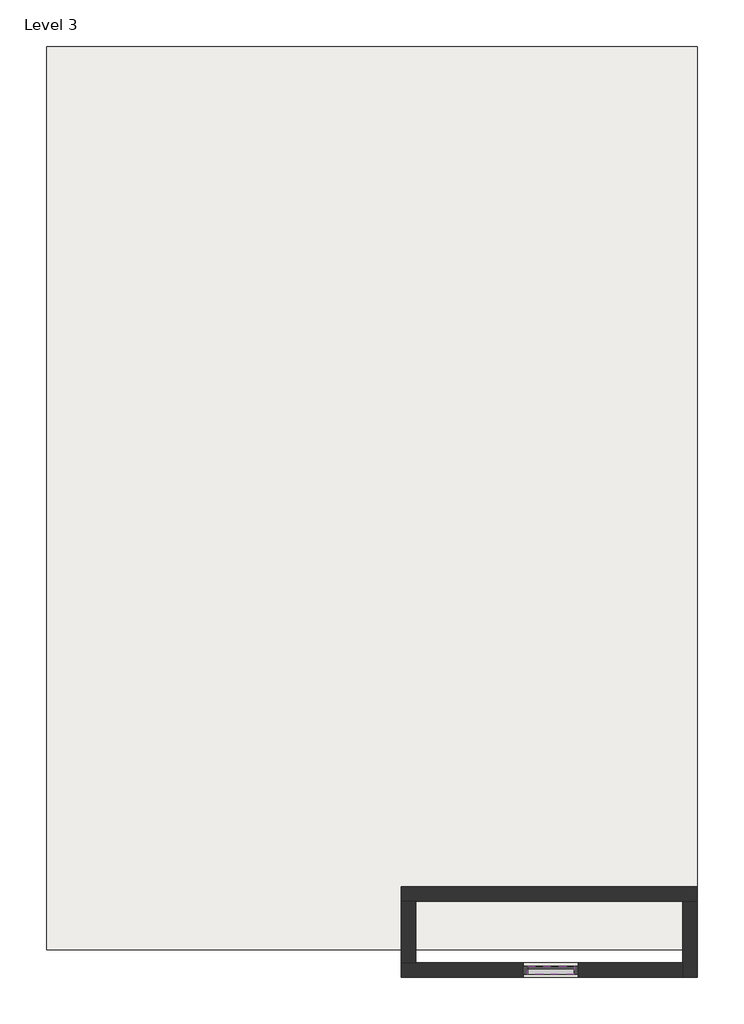
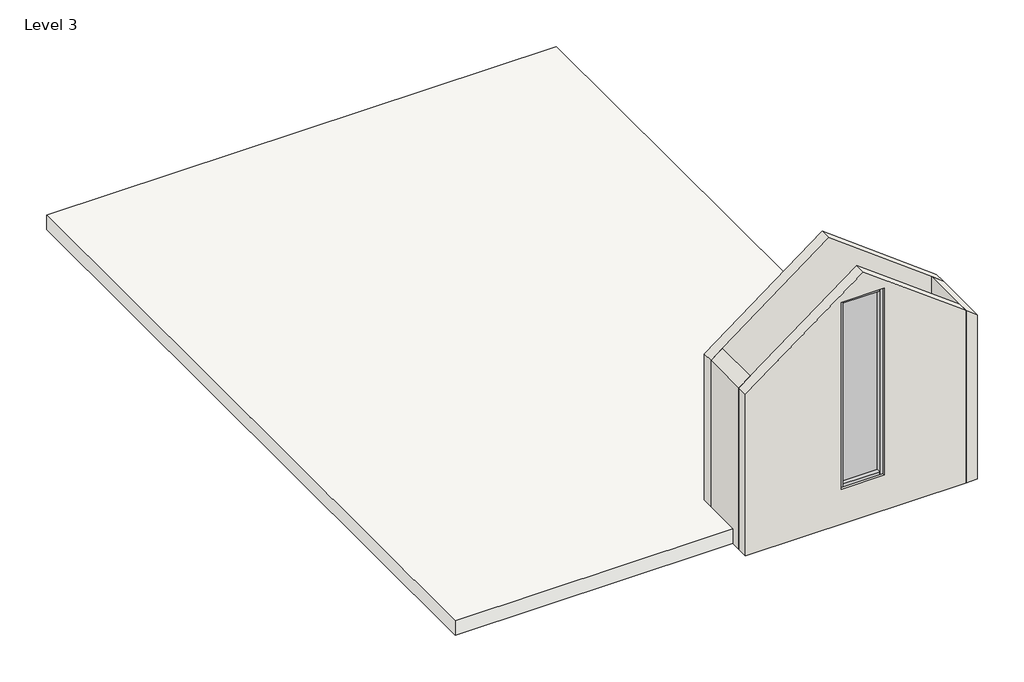
# One storey: 4 members, 4 walls, 1 plate, 1 roof.
"""IFC4 building model written with IfcOpenShell, lengths in millimetres."""

from ifc_helpers import new_model, si_unit, frame, origin, place, context, project, spatial, polyline, outline, extrude, faceted_brep, transform, mapped, element, save
from components import member_b91b5e2d, member_3472e6fb, system_panel_glazed_5544ac81

model = new_model("IFC4")

# Units and contexts
model_context = context("Model", 3, world=origin())
ifc_project = project(units=[si_unit("LENGTHUNIT", "METRE", prefix="MILLI")], contexts=[model_context])

# Site, building, storey
site = spatial("IfcSite", under=ifc_project)
building = spatial("IfcBuilding", under=site)
storey = spatial("IfcBuildingStorey", under=building, Name="Level 3", Elevation=6096.0)

# Members
placement = place(None, origin())
member_shape = member_b91b5e2d(model_context)
element("IfcMember", 1, ObjectType="Rectangular Mullion : 2.5\" x 5\" rectangular", at=placement, inside=storey, context=model_context, shape_type="MappedRepresentation", body=[
    mapped(member_shape, transform((-9357.9624893, -13304.7040375, 10789.859026), x_axis=(0.0, 0.0, 1.0), y_axis=(0.0, -1.0, 0.0), z_axis=(1.0, 0.0, 0.0))),
])
element("IfcMember", 2, ObjectType="Rectangular Mullion : 2.5\" x 5\" rectangular", at=placement, inside=storey, context=model_context, shape_type="MappedRepresentation", body=[
    mapped(member_shape, transform((-10092.3642918, -13304.7040375, 6829.7980932), x_axis=(0.0, 0.0, -1.0), y_axis=(0.0, -1.0, 0.0), z_axis=(-1.0, 0.0, 0.0))),
])
member_2_shape = member_3472e6fb(model_context)
element("IfcMember", 3, ObjectType="Rectangular Mullion : 2.5\" x 5\" rectangular", at=placement, inside=storey, context=model_context, shape_type="MappedRepresentation", body=[
    mapped(member_2_shape, transform((-10155.8642918, -13304.7040375, 10789.859026), x_axis=(-1.0, 0.0, 0.0), y_axis=(0.0, -1.0, 0.0), z_axis=(0.0, 0.0, 1.0))),
])
element("IfcMember", 4, ObjectType="Rectangular Mullion : 2.5\" x 5\" rectangular", at=placement, inside=storey, context=model_context, shape_type="MappedRepresentation", body=[
    mapped(member_2_shape, transform((-9294.4624893, -13304.7040375, 6829.7980932), x_axis=(1.0, 0.0, 0.0), y_axis=(0.0, -1.0, 0.0), z_axis=(0.0, 0.0, -1.0))),
])

# Plate
system_panel_glazed_shape = system_panel_glazed_5544ac81(model_context)
element("IfcPlate", 5, ObjectType="System Panel : Glazed", at=placement, inside=storey, context=model_context, shape_type="MappedRepresentation", body=[
    mapped(system_panel_glazed_shape, transform((-9725.1633906, -13304.7040375, 6893.2980932), x_axis=(1.0, 0.0, 0.0), y_axis=(0.0, 1.0, 0.0), z_axis=(0.0, 0.0, 1.0))),
])

# Roof
element("IfcRoof", 6, ObjectType="Generic - 12\"", at=placement, inside=storey, context=model_context, shape_type="SweptSolid", body=[
    extrude(outline(polyline([(-17638.3624893, 1185.9959625), (-7427.5624893, 1185.9959625), (-7427.5624893, -12987.2040375), (-17638.3624893, -12987.2040375), (-17638.3624893, 1185.9959625)])), frame((0.0, 0.0, 6096.0), z_axis=(0.0, 0.0, 1.0), x_axis=(1.0, 0.0, 0.0)), (0.0, 0.0, 1.0), 304.8),
])

# Walls
element("IfcWall", 7, ObjectType="9\"", at=placement, inside=storey, context=model_context, shape_type="Brep", body=[
    faceted_brep([(-12073.5642918, -12225.2040375, 6096.0), (-11844.9642918, -12225.2040375, 6096.0), (-7656.1624893, -12225.2040375, 6096.0), (-7427.5624893, -12225.2040375, 6096.0), (-7427.5624893, -12225.2040375, 9567.0103984), (-7656.1624893, -12225.2040375, 9738.4603984), (-9712.3774133, -12225.2040375, 11280.6215913), (-11844.9642918, -12225.2040375, 9681.1814324), (-12073.5642918, -12225.2040375, 9509.7314324), (-12073.5642918, -11996.6040375, 6096.0), (-12073.5642918, -11996.6040375, 9509.7314324), (-9712.3774133, -11996.6040375, 11280.6215913), (-7427.5624893, -11996.6040375, 9567.0103984), (-7427.5624893, -11996.6040375, 6096.0)], [[[0, 1, 2, 3, 4, 5, 6, 7, 8]], [[9, 10, 11, 12, 13]], [[3, 2, 1, 0, 9, 13]], [[4, 3, 13, 12]], [[0, 8, 10, 9]], [[8, 7, 6, 11, 10]], [[6, 5, 4, 12, 11]]]),
])
element("IfcWall", 8, ObjectType="9\"", at=placement, inside=storey, context=model_context, shape_type="Brep", body=[
    faceted_brep([(-7656.1624893, -12225.2040375, 6096.0), (-7656.1624893, -13190.4040375, 6096.0), (-7656.1624893, -13419.0040375, 6096.0), (-7656.1624893, -13419.0040375, 9738.4603984), (-7656.1624893, -13190.4040375, 9738.4603984), (-7656.1624893, -12225.2040375, 9738.4603984), (-7427.5624893, -12225.2040375, 6096.0), (-7427.5624893, -12225.2040375, 9567.0103984), (-7427.5624893, -13419.0040375, 9567.0103984), (-7427.5624893, -13419.0040375, 6096.0)], [[[0, 1, 2, 3, 4, 5]], [[6, 7, 8, 9]], [[2, 1, 0, 6, 9]], [[0, 5, 7, 6]], [[3, 2, 9, 8]], [[5, 4, 3, 8, 7]]]),
])
element("IfcWall", 9, ObjectType="9\"", at=placement, inside=storey, context=model_context, shape_type="Brep", body=[
    faceted_brep([(-7656.1624893, -13190.4040375, 6096.0), (-11844.9642918, -13190.4040375, 6096.0), (-12073.5642918, -13190.4040375, 6096.0), (-12073.5642918, -13190.4040375, 9509.7314324), (-11844.9642918, -13190.4040375, 9681.1814324), (-9712.3774133, -13190.4040375, 11280.6215913), (-7656.1624893, -13190.4040375, 9738.4603984), (-10155.8642918, -13190.4040375, 10789.859026), (-10155.8642918, -13190.4040375, 6829.7980932), (-9294.4624893, -13190.4040375, 6829.7980932), (-9294.4624893, -13190.4040375, 10789.859026), (-12073.5642918, -13419.0040375, 6096.0), (-7656.1624893, -13419.0040375, 6096.0), (-7656.1624893, -13419.0040375, 9738.4603984), (-9712.3774133, -13419.0040375, 11280.6215913), (-12073.5642918, -13419.0040375, 9509.7314324), (-10155.8642918, -13419.0040375, 6829.7980932), (-10155.8642918, -13419.0040375, 10789.859026), (-9294.4624893, -13419.0040375, 10789.859026), (-9294.4624893, -13419.0040375, 6829.7980932)], [[[0, 1, 2, 3, 4, 5, 6], [7, 8, 9, 10]], [[11, 12, 13, 14, 15], [16, 17, 18, 19]], [[2, 1, 0, 12, 11]], [[0, 6, 13, 12]], [[3, 2, 11, 15]], [[13, 6, 5, 14]], [[3, 15, 14, 5, 4]], [[16, 8, 7, 17]], [[17, 7, 10, 18]], [[18, 10, 9, 19]], [[8, 16, 19, 9]]]),
])
element("IfcWall", 10, ObjectType="9\"", at=placement, inside=storey, context=model_context, shape_type="SweptSolid", body=[
    extrude(outline(polyline([(9509.7314324, -12073.5642918), (6096.0, -12073.5642918), (6096.0, -11844.9642918), (9681.1814324, -11844.9642918), (9509.7314324, -12073.5642918)])), frame((0.0, -13190.4040375, 0.0), z_axis=(0.0, 1.0, 0.0), x_axis=(0.0, 0.0, 1.0)), (0.0, 0.0, 1.0), 965.2),
])

save(model, "model.ifc")

# Revit data of these elements
# Type "Rectangular Mullion : 2.5\" x 5\" rectangular"
#   built-in parameter 1007304 = 0.416667 (stored number, unit not read)
#   built-in parameter 1007301 = 0.104167 (stored number, unit not read)
#   built-in parameter 1007300 = 0.104167 (stored number, unit not read)
# Type "System Panel : Glazed"
#   Construction Type Id = "GSP4R"
#   Analytic Construction = "1/8 in Pilkington single glazing"
#   Visual Light Transmittance = 0.9
#   Solar Heat Gain Coefficient = 0.86
#   Heat Transfer Coefficient (U) = 1.18115 BTU/(h·ft²·°F)
#   Define Thermal Properties by = 1
# Type "Generic - 12\""
#   Assembly Code = "B1020"
#   Layers, outside or top first: 1' - 0" no material (function 1)
# Type "9\""
#   Assembly Code = "B2010"
#   Layers, outside or top first: 0' - 9" no material (function 1)
# Elements 1, 2, 3, 4 (IfcMember, "Rectangular Mullion : 2.5\" x 5\" rectangular")
#   Phase Created = New Construction
#   Materials on its faces: "Aluminum"
# Element 5 (IfcPlate, "System Panel : Glazed")
#   Phase Created = New Construction
#   Materials on its faces: "Glass"
# Element 6 (IfcRoof, "Generic - 12\"")
#   built-in parameter 1001705 = 21 (stored number, unit not read)
#   built-in parameter 1001710 = 33615
#   Phase Created = New Construction
#   Materials on its faces: "Default Roof"
# Elements 7, 8, 9, 10 (IfcWall, "9\"")
#   Top Offset = 0' - 0"
#   Base Offset = 0' - 0"
#   Unconnected Height = 10' - 0"
#   wall height = 10' - 0"
#   Phase Created = New Construction
#   Base Constraint = Level 3
#   Materials on its faces: "Default Wall"
# Materials
#   "Aluminum": class "Metal", colour RGB 247 247 247, transparency 0, Description = "Aluminum 6061", Cost = 0
#   "Glass": class "Glass", colour RGB 0 128 192, transparency 0.75, Description = "Soda Lime Glass", Cost = 0
#   "Default Roof": colour RGB 88 101 114, transparency 0, Cost = 0
#   "Default Wall": colour RGB 128 128 128, transparency 0, Cost = 0
